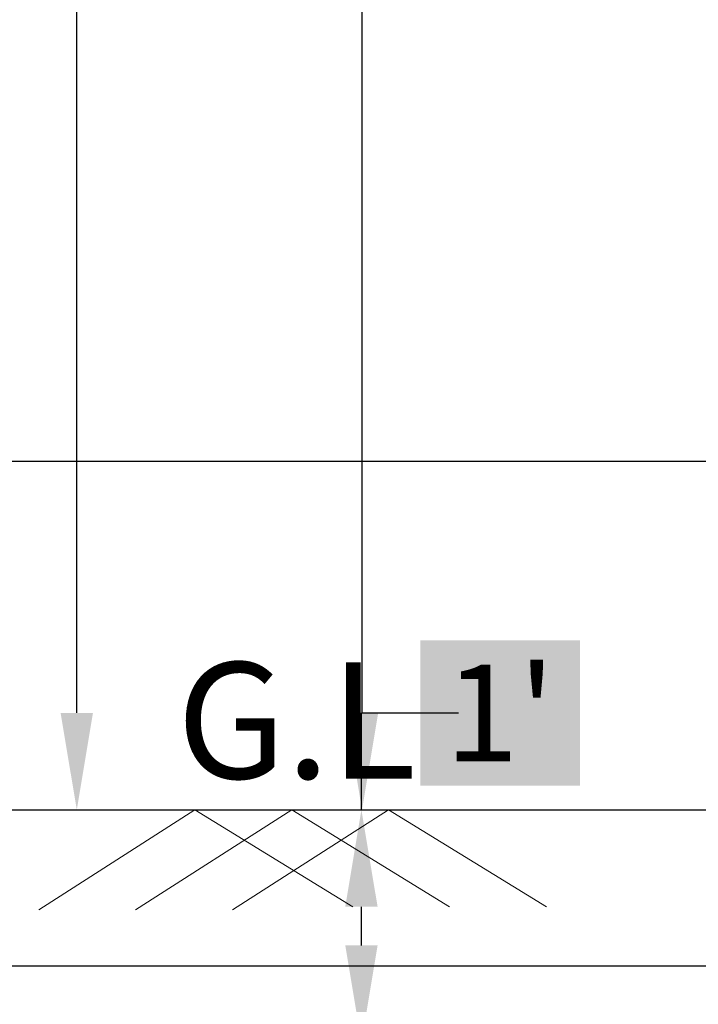
# Model space of a CAD drawing. Units: inches. Extents: x -301 to 715, y -607 to 364.
# Tile 36 of 141: x 159 to 194, y -492 to -441. Entities that reach past the tile are written whole.
import ezdxf

# ---------------------------------------------------------------- set-up
doc = ezdxf.new("R2010")
doc.units = ezdxf.units.IN
doc.header["$MEASUREMENT"] = 0
for name, color, linetype, lineweight in [('A-ANNO-DIMS', 2, 'Continuous', 18), ('A-ANNO-SYMB', 4, 'Continuous', 18), ('A-GRND', 7, 'Continuous', 25)]:
    doc.layers.add(name, color=color, linetype=linetype, lineweight=lineweight)
doc.styles.get("Standard").update_dxf_attribs({"font": 'arial.ttf'})
doc.dimstyles.get("Standard").update_dxf_attribs({"dimtxt": 0.18, "dimasz": 0.18, "dimexe": 0.18, "dimexo": 0.0625, "dimgap": 0.09, "dimtad": 0, "dimtih": 1, "dimtoh": 1, "dimdec": 1, "dimzin": 0, "dimdsep": 46, "dimlunit": 4, "dimtxsty": 'Standard', "dimcen": 0.09, "dimclrd": 3, "dimclre": 4, "dimclrt": 6, "dimadec": 0, "dimazin": 0, "dimtfac": 1, "dimtdec": 1, "dimtofl": 0, "dimtmove": 0, "dimatfit": 3, "dimfxl": 1, "dimtfill": 2, "dimtfillclr": 51, "dimtolj": 1, "dimtzin": 0, "dimarcsym": 0})

# ---------------------------------------------------------------- blocks, each defined once
blk = doc.blocks.new('*D76')
at = {"layer": 'A-ANNO-DIMS', "color": 0, "lineweight": -2, "transparency": 16777216}
for p, q in [((158.28, -324.519), (162.311, -324.519)), ((162.131, -329.519), (162.131, -400.354)), ((162.131, -476.477), (162.131, -405.643)), ((158.28, -481.477), (162.311, -481.477))]:
    blk.add_line(p, q, dxfattribs=at)
at = {"layer": 'A-ANNO-DIMS', "color": 0, "transparency": 16777216}
for points in [[(161.297, -329.519), (162.964, -329.519), (162.131, -324.519)], [(161.297, -476.477), (162.964, -476.477), (162.131, -481.477)]]:
    blk.add_solid(points, dxfattribs=at)
at = {"layer": 'Defpoints', "color": 0, "transparency": 16777216}
for p in [(158.218, -324.519), (162.131, -324.519), (158.218, -481.477)]:
    blk.add_point(p, dxfattribs=at)
at = {"layer": 'A-ANNO-DIMS', "color": 0, "transparency": 16777216, "insert": (162.131, -402.998), "char_height": 5, "attachment_point": 5, "bg_fill": 1, "box_fill_scale": 1.25, "bg_fill_color": 51, "bg_fill_transparency": 0}
blk.add_mtext('\\A1;13\'-1"', dxfattribs=at)
blk = doc.blocks.new('*D80')
at = {"layer": 'A-ANNO-DIMS', "color": 0, "lineweight": -2, "transparency": 16777216}
for p, q in [((176.814, -481.477), (176.814, -476.477)), ((176.814, -476.477), (181.814, -476.477)), ((153.318, -481.477), (176.994, -481.477)), ((176.814, -488.477), (176.814, -486.477)), ((153.318, -493.477), (176.994, -493.477))]:
    blk.add_line(p, q, dxfattribs=at)
at = {"layer": 'A-ANNO-DIMS', "color": 0, "transparency": 16777216}
for points in [[(175.981, -486.477), (177.648, -486.477), (176.814, -481.477)], [(175.981, -488.477), (177.648, -488.477), (176.814, -493.477)]]:
    blk.add_solid(points, dxfattribs=at)
at = {"layer": 'Defpoints', "color": 0, "transparency": 16777216}
for p in [(153.255, -481.477), (176.814, -481.477), (153.255, -493.477)]:
    blk.add_point(p, dxfattribs=at)
at = {"layer": 'A-ANNO-DIMS', "color": 0, "transparency": 16777216, "insert": (183.969, -476.477), "char_height": 5, "attachment_point": 5, "bg_fill": 1, "box_fill_scale": 1.25, "bg_fill_color": 51, "bg_fill_transparency": 0}
blk.add_mtext("\\A1;1'", dxfattribs=at)
blk = doc.blocks.new('*D81')
at = {"layer": 'A-ANNO-DIMS', "color": 0, "lineweight": -2, "transparency": 16777216}
for p, q in [((155.28, -385.477), (177.024, -385.477)), ((176.844, -390.477), (176.844, -430.835)), ((176.844, -476.477), (176.844, -436.12)), ((158.28, -481.477), (177.024, -481.477))]:
    blk.add_line(p, q, dxfattribs=at)
at = {"layer": 'A-ANNO-DIMS', "color": 0, "transparency": 16777216}
for points in [[(176.011, -390.477), (177.678, -390.477), (176.844, -385.477)], [(176.011, -476.477), (177.678, -476.477), (176.844, -481.477)]]:
    blk.add_solid(points, dxfattribs=at)
at = {"layer": 'Defpoints', "color": 0, "transparency": 16777216}
for p in [(155.218, -385.477), (158.218, -481.477), (176.844, -481.477)]:
    blk.add_point(p, dxfattribs=at)
at = {"layer": 'A-ANNO-DIMS', "color": 0, "transparency": 16777216, "insert": (176.844, -433.477), "char_height": 5, "attachment_point": 5, "bg_fill": 1, "box_fill_scale": 1.25, "bg_fill_color": 51, "bg_fill_transparency": 0}
blk.add_mtext("\\A1;8'", dxfattribs=at)
blk = doc.blocks.new('GRADE-MARK-3')
for p, q in [((8.051, 5.162), (0, 0)), ((13.051, 5.162), (5, 0)), ((8.051, 5.162), (16.197, 0.151)), ((18.051, 5.162), (10, 0)), ((13.051, 5.162), (21.197, 0.151)), ((18.051, 5.162), (26.197, 0.151))]:
    blk.add_line(p, q)
blk = doc.blocks.new('*D176')
at = {"layer": 'A-ANNO-DIMS', "color": 4, "lineweight": -2, "transparency": 16777216}
for p, q in [((148.28, -324.477), (215.605, -324.477)), ((-15.22, -540.477), (215.605, -540.477))]:
    blk.add_line(p, q, dxfattribs=at)
at = {"layer": 'A-ANNO-DIMS', "color": 3, "lineweight": -2, "transparency": 16777216}
for p, q in [((215.425, -324.657), (215.425, -432.296)), ((215.425, -540.297), (215.425, -432.659))]:
    blk.add_line(p, q, dxfattribs=at)
at = {"layer": 'A-ANNO-DIMS', "color": 3, "transparency": 16777216}
for points in [[(215.395, -324.657), (215.455, -324.657), (215.425, -324.477)], [(215.395, -540.297), (215.455, -540.297), (215.425, -540.477)]]:
    blk.add_solid(points, dxfattribs=at)
at = {"layer": 'Defpoints', "color": 0, "transparency": 16777216}
for p in [(148.218, -324.477), (-15.282, -540.477), (215.425, -540.477)]:
    blk.add_point(p, dxfattribs=at)
at = {"layer": 'A-ANNO-DIMS', "color": 6, "transparency": 16777216, "insert": (215.425, -432.477), "char_height": 0.18, "attachment_point": 5, "bg_fill": 1, "box_fill_scale": 1.25, "bg_fill_color": 51, "bg_fill_transparency": 0}
blk.add_mtext('\\A1;18\'-0"', dxfattribs=at)
blk = doc.blocks.new('*D188')
at = {"layer": 'A-ANNO-DIMS', "color": 4, "lineweight": -2, "transparency": 16777216}
for p, q in [((148.28, -463.477), (215.605, -463.477)), ((158.28, -481.477), (215.605, -481.477))]:
    blk.add_line(p, q, dxfattribs=at)
at = {"layer": 'A-ANNO-DIMS', "color": 3, "lineweight": -2, "transparency": 16777216}
for p, q in [((215.425, -463.657), (215.425, -472.296)), ((215.425, -481.297), (215.425, -472.659))]:
    blk.add_line(p, q, dxfattribs=at)
at = {"layer": 'A-ANNO-DIMS', "color": 3, "transparency": 16777216}
for points in [[(215.395, -463.657), (215.455, -463.657), (215.425, -463.477)], [(215.395, -481.297), (215.455, -481.297), (215.425, -481.477)]]:
    blk.add_solid(points, dxfattribs=at)
at = {"layer": 'Defpoints', "color": 0, "transparency": 16777216}
for p in [(148.218, -463.477), (215.425, -463.477), (158.218, -481.477)]:
    blk.add_point(p, dxfattribs=at)
at = {"layer": 'A-ANNO-DIMS', "color": 6, "transparency": 16777216, "insert": (215.425, -472.477), "char_height": 0.18, "attachment_point": 5, "bg_fill": 1, "box_fill_scale": 1.25, "bg_fill_color": 51, "bg_fill_transparency": 0}
blk.add_mtext('\\A1;1\'-6"', dxfattribs=at)
blk = doc.blocks.new('*D200')
at = {"layer": 'A-ANNO-DIMS', "color": 4, "lineweight": -2, "transparency": 16777216}
for p, q in [((412.955, -393.552), (121.926, -393.552)), ((412.955, -489.552), (121.926, -489.552))]:
    blk.add_line(p, q, dxfattribs=at)
at = {"layer": 'A-ANNO-DIMS', "color": 3, "lineweight": -2, "transparency": 16777216}
for p, q in [((122.106, -393.732), (122.106, -441.371)), ((122.106, -489.372), (122.106, -441.734))]:
    blk.add_line(p, q, dxfattribs=at)
at = {"layer": 'A-ANNO-DIMS', "color": 3, "transparency": 16777216}
for points in [[(122.076, -393.732), (122.136, -393.732), (122.106, -393.552)], [(122.076, -489.372), (122.136, -489.372), (122.106, -489.552)]]:
    blk.add_solid(points, dxfattribs=at)
at = {"layer": 'Defpoints', "color": 0, "transparency": 16777216}
for p in [(122.106, -393.552), (413.018, -393.552), (413.018, -489.552)]:
    blk.add_point(p, dxfattribs=at)
at = {"layer": 'A-ANNO-DIMS', "color": 6, "transparency": 16777216, "insert": (122.106, -441.552), "char_height": 0.18, "attachment_point": 5, "bg_fill": 1, "box_fill_scale": 1.25, "bg_fill_color": 51, "bg_fill_transparency": 0}
blk.add_mtext('\\A1;8\'-0"', dxfattribs=at)

msp = doc.modelspace()

# ---------------------------------------------------------------- linework, layer by layer
at = {"layer": 'A-GRND'}
msp.add_line((155.218, -481.477), (191.218, -481.477), dxfattribs=at)

# ---------------------------------------------------------------- block references
at = {"layer": 'A-ANNO-SYMB'}
msp.add_blockref('GRADE-MARK-3', (160.167, -486.639), dxfattribs=at)

# ---------------------------------------------------------------- texts
msp.add_text('G.L', height=6, dxfattribs=at).set_placement((167.28, -479.862))

# ---------------------------------------------------------------- dimensions: what is measured, and where the dimension line sits
at = {"layer": 'A-ANNO-DIMS'}
for base, p1, p2, override, picture, middle in [((215.425, -540.477), (148.218, -324.477), (-15.282, -540.477), {"dimdec": 1, "dimlfac": 1, "dimrnd": 0, "dimzin": 1, "dimdsep": 46, "dimlunit": 4, "dimfrac": 2}, '*D176', (215.425, -432.477)), ((162.131, -324.519), (158.218, -481.477), (158.218, -324.519), {"dimtxt": 5, "dimasz": 5, "dimclrd": 0, "dimclre": 0, "dimclrt": 0}, '*D76', (162.131, -402.998)), ((176.844, -481.477), (155.218, -385.477), (158.218, -481.477), {"dimtxt": 5, "dimasz": 5, "dimclrd": 0, "dimclre": 0, "dimclrt": 0}, '*D81', (176.844, -433.477)), ((122.106, -393.552), (413.018, -489.552), (413.018, -393.552), {"dimdec": 1, "dimlfac": 1, "dimrnd": 0, "dimzin": 1, "dimdsep": 46, "dimlunit": 4, "dimfrac": 2}, '*D200', (122.106, -441.552)), ((215.425, -463.477), (158.218, -481.477), (148.218, -463.477), {"dimdec": 1, "dimlfac": 1, "dimrnd": 0, "dimzin": 1, "dimdsep": 46, "dimlunit": 4, "dimfrac": 2}, '*D188', (215.425, -472.477)), ((176.814, -481.477), (153.255, -493.477), (153.255, -481.477), {"dimtxt": 5, "dimasz": 5, "dimclrd": 0, "dimclre": 0, "dimclrt": 0}, '*D80', (183.969, -476.477))]:
    dim = msp.add_linear_dim(base=base, p1=p1, p2=p2, angle=90, dimstyle='Standard', override=override, dxfattribs=at)
    dim.commit()
    dim.dimension.update_dxf_attribs({"geometry": picture, "text_midpoint": middle})

doc.saveas('drawing.dxf')
